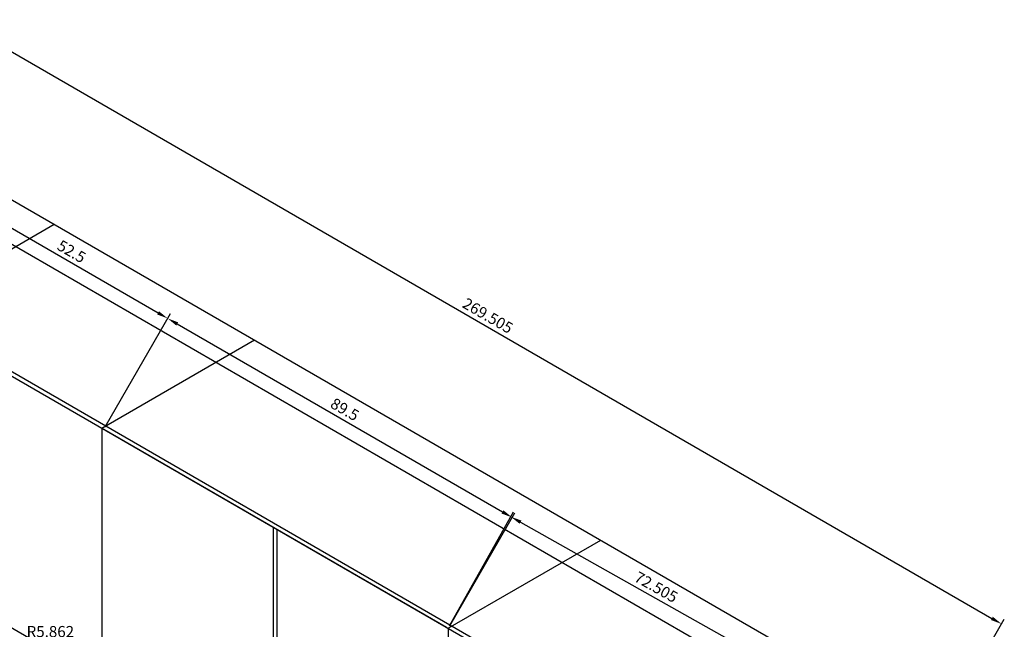
# Model space of a CAD drawing. Units: centimetres. Extents: x 239489 to 240034, y 95136 to 95693.
# Tile 4 of 4: x 239762 to 239984, y 95556 to 95693. Entities that reach past the tile are written whole.
import ezdxf

# ---------------------------------------------------------------- set-up
doc = ezdxf.new("R2010")
doc.units = ezdxf.units.CM
doc.layers.add('A-ANNO-DIMS', color=2, linetype='Continuous', lineweight=18)
doc.layers.add('A-FLOR-CASE', color=7, linetype='Continuous', lineweight=25)
doc.styles.get("Standard").update_dxf_attribs({"font": 'arial.ttf'})
doc.dimstyles.new('ISO-25', dxfattribs={"dimtxt": 2.5, "dimasz": 2.5, "dimexe": 1.25, "dimexo": 0.625, "dimtad": 1, "dimdec": 1, "dimdsep": 46, "dimtxsty": 'Standard', "dimcen": 2.5, "dimadec": 0, "dimazin": 0, "dimtfac": 1, "dimtdec": 1, "dimtmove": 0, "dimatfit": 3, "dimfxl": 1, "dimarcsym": 0})

# ---------------------------------------------------------------- blocks, each defined once
blk = doc.blocks.new('*D5')
at = {"layer": 'A-ANNO-DIMS', "color": 0, "lineweight": -2, "transparency": 16777216}
for p, q in [((239735.57, 95667.89), (239750.25, 95693.33)), ((239751.79, 95691), (239980.86, 95558.75)), ((239968.97, 95533.14), (239983.65, 95558.58))]:
    blk.add_line(p, q, dxfattribs=at)
at = {"layer": 'A-ANNO-DIMS', "color": 0, "transparency": 16777216}
for points in [[(239752, 95691.36), (239751.59, 95690.64), (239749.63, 95692.25)], [(239981.07, 95559.11), (239980.65, 95558.39), (239983.03, 95557.5)]]:
    blk.add_solid(points, dxfattribs=at)
at = {"layer": 'Defpoints', "color": 0, "transparency": 16777216}
for p in [(239735.25, 95667.35), (239983.03, 95557.5), (239968.65, 95532.6)]:
    blk.add_point(p, dxfattribs=at)
at = {"layer": 'A-ANNO-DIMS', "color": 0, "transparency": 16777216, "insert": (239867.28, 95626.52), "char_height": 2.5, "attachment_point": 5, "rotation": 330}
blk.add_mtext('269.505', dxfattribs=at)
blk = doc.blocks.new('*D22')
at = {"layer": 'A-ANNO-DIMS', "color": 0, "lineweight": -2, "transparency": 16777216}
for p, q in [((239735.88, 95628.07), (239750.57, 95653.51)), ((239752.11, 95651.18), (239793.24, 95627.43)), ((239781.35, 95601.82), (239796.03, 95627.26))]:
    blk.add_line(p, q, dxfattribs=at)
at = {"layer": 'A-ANNO-DIMS', "color": 0, "transparency": 16777216}
for points in [[(239752.32, 95651.54), (239751.9, 95650.82), (239749.94, 95652.43)], [(239793.45, 95627.79), (239793.04, 95627.07), (239795.41, 95626.18)]]:
    blk.add_solid(points, dxfattribs=at)
at = {"layer": 'Defpoints', "color": 0, "transparency": 16777216}
for p in [(239735.57, 95627.53), (239795.41, 95626.18), (239781.03, 95601.28)]:
    blk.add_point(p, dxfattribs=at)
at = {"layer": 'A-ANNO-DIMS', "color": 0, "transparency": 16777216, "insert": (239773.63, 95640.95), "char_height": 2.5, "attachment_point": 5, "rotation": 330}
blk.add_mtext('52.5', dxfattribs=at)
blk = doc.blocks.new('*D23')
at = {"layer": 'A-ANNO-DIMS', "color": 0, "lineweight": -2, "transparency": 16777216}
for p, q in [((239781.35, 95601.82), (239796.03, 95627.26)), ((239797.57, 95624.93), (239870.75, 95582.68)), ((239858.86, 95557.07), (239873.54, 95582.51))]:
    blk.add_line(p, q, dxfattribs=at)
at = {"layer": 'A-ANNO-DIMS', "color": 0, "transparency": 16777216}
for points in [[(239797.78, 95625.29), (239797.37, 95624.57), (239795.41, 95626.18)], [(239870.96, 95583.04), (239870.54, 95582.32), (239872.92, 95581.43)]]:
    blk.add_solid(points, dxfattribs=at)
at = {"layer": 'Defpoints', "color": 0, "transparency": 16777216}
for p in [(239781.03, 95601.28), (239872.92, 95581.43), (239858.54, 95556.53)]:
    blk.add_point(p, dxfattribs=at)
at = {"layer": 'A-ANNO-DIMS', "color": 0, "transparency": 16777216, "insert": (239835.11, 95605.45), "char_height": 2.5, "attachment_point": 5, "rotation": 330}
blk.add_mtext('89.5', dxfattribs=at)
blk = doc.blocks.new('*D24')
at = {"layer": 'A-ANNO-DIMS', "color": 0, "lineweight": -2, "transparency": 16777216}
for p, q in [((239858.85, 95557.08), (239873.23, 95582.69)), ((239874.8, 95580.37), (239933.66, 95547.32)), ((239922.07, 95521.58), (239936.45, 95547.19))]:
    blk.add_line(p, q, dxfattribs=at)
at = {"layer": 'A-ANNO-DIMS', "color": 0, "transparency": 16777216}
for points in [[(239875, 95580.74), (239874.6, 95580.01), (239872.62, 95581.6)], [(239933.86, 95547.69), (239933.46, 95546.96), (239935.84, 95546.1)]]:
    blk.add_solid(points, dxfattribs=at)
at = {"layer": 'Defpoints', "color": 0, "transparency": 16777216}
for p in [(239858.54, 95556.53), (239935.84, 95546.1), (239921.76, 95521.03)]:
    blk.add_point(p, dxfattribs=at)
at = {"layer": 'A-ANNO-DIMS', "color": 0, "transparency": 16777216, "insert": (239905.16, 95565.51), "char_height": 2.5, "attachment_point": 5, "rotation": 330.6844}
blk.add_mtext('72.505', dxfattribs=at)
blk = doc.blocks.new('*D39')
at = {"layer": 'A-ANNO-DIMS', "color": 0, "lineweight": -2, "transparency": 16777216}
for p, q in [((239717.29, 95549.03), (239731.97, 95574.47)), ((239733.51, 95572.13), (239765.51, 95553.66)), ((239753.61, 95528.06), (239768.3, 95553.5))]:
    blk.add_line(p, q, dxfattribs=at)
at = {"layer": 'A-ANNO-DIMS', "color": 0, "transparency": 16777216}
for points in [[(239733.72, 95572.5), (239733.31, 95571.77), (239731.35, 95573.38)], [(239765.72, 95554.02), (239765.3, 95553.3), (239767.67, 95552.41)]]:
    blk.add_solid(points, dxfattribs=at)
at = {"layer": 'Defpoints', "color": 0, "transparency": 16777216}
for p in [(239767.67, 95552.41), (239716.97, 95548.49), (239753.3, 95527.52)]:
    blk.add_point(p, dxfattribs=at)
at = {"layer": 'A-ANNO-DIMS', "color": 0, "transparency": 16777216, "insert": (239750.46, 95564.55), "char_height": 2.5, "attachment_point": 5, "rotation": 330}
blk.add_mtext('41.943', dxfattribs=at)
blk = doc.blocks.new('*D51')
at = {"layer": 'A-ANNO-DIMS', "color": 0, "lineweight": -2, "transparency": 16777216}
for p, q in [((239762.99, 95553.56), (239777.54, 95553.56)), ((239785.9, 95553.56), (239780.04, 95553.56))]:
    blk.add_line(p, q, dxfattribs=at)
at = {"layer": 'A-ANNO-DIMS', "color": 0, "transparency": 16777216}
blk.add_solid([(239777.54, 95553.98), (239777.54, 95553.15), (239780.04, 95553.56)], dxfattribs=at)
at = {"layer": 'Defpoints', "color": 0, "transparency": 16777216}
for p in [(239780.04, 95553.56), (239785.9, 95553.56)]:
    blk.add_point(p, dxfattribs=at)
at = {"layer": 'A-ANNO-DIMS', "color": 0, "transparency": 16777216, "insert": (239769.01, 95555.46), "char_height": 2.5, "attachment_point": 5, "rotation": 0.0036}
blk.add_mtext('R5.862', dxfattribs=at)

msp = doc.modelspace()

# ---------------------------------------------------------------- linework, layer by layer
at = {"layer": 'A-FLOR-CASE'}
for p, q in [((239735.2548, 95667.3502), (239968.6531, 95532.5976)), ((239735.2548, 95657.3502), (239947.431, 95534.8502)), ((239736.4333, 95628.0306), (239769.8958, 95647.3502)), ((239735.5673, 95628.5306), (239921.7628, 95521.0306)), ((239735.5673, 95627.5306), (239921.7628, 95520.0306)), ((239780.6006, 95601.5306), (239814.9291, 95621.3502)), ((239780.6006, 95601.5306), (239780.6006, 95538.5306)), ((239781.0336, 95601.2806), (239858.1099, 95556.7806)), ((239819.1388, 95579.2806), (239819.1388, 95533.8134)), ((239820.0048, 95578.7806), (239820.0048, 95533.3134)), ((239858.5429, 95556.5306), (239892.8714, 95576.3502)), ((239858.5429, 95556.5306), (239858.5429, 95493.5306))]:
    msp.add_line(p, q, dxfattribs=at)

# ---------------------------------------------------------------- dimensions: what is measured, and where the dimension line sits
at = {"layer": 'A-ANNO-DIMS'}
for base, p1, p2, angle, override, picture, middle in [((239983.0281, 95557.4959), (239735.2548, 95667.3502), (239968.6531, 95532.5976), 330, {"dimdec": 3, "dimlfac": 1, "dimrnd": 0, "dimzin": 0, "dimdsep": 46, "dimlunit": 2}, '*D5', (239867.2796, 95626.5188)), ((239795.4086, 95626.1788), (239735.5673, 95627.5306), (239781.0336, 95601.2806), 330, {"dimdec": 1, "dimlfac": 1, "dimrnd": 0, "dimzin": 0, "dimdsep": 46, "dimlunit": 2}, '*D22', (239773.6262, 95640.9505)), ((239872.9179, 95581.4288), (239781.0336, 95601.2806), (239858.5429, 95556.5306), 330, {"dimdec": 1, "dimlfac": 1, "dimrnd": 0, "dimzin": 0, "dimdsep": 46, "dimlunit": 2}, '*D23', (239835.114, 95605.4505)), ((239935.8394, 95546.0987), (239858.5429, 95556.5306), (239921.7628, 95521.0306), 330.684376, {"dimdec": 3, "dimlfac": 1, "dimrnd": 0, "dimzin": 0, "dimdsep": 46, "dimlunit": 2}, '*D24', (239905.1604, 95565.5067)), ((239767.673, 95552.4136), (239716.9746, 95548.4867), (239753.298, 95527.5153), 330, {"dimdec": 3, "dimlfac": 1, "dimrnd": 0, "dimzin": 0, "dimdsep": 46, "dimlunit": 2}, '*D39', (239750.4624, 95564.5466))]:
    dim = msp.add_linear_dim(base=base, p1=p1, p2=p2, angle=angle, dimstyle='ISO-25', override=override, dxfattribs=at)
    dim.commit()
    dim.dimension.update_dxf_attribs({"geometry": picture, "text_midpoint": middle})
dim = msp.add_radius_dim(center=(239785.9025, 95553.5634), mpoint=(239780.0408, 95553.563), dimstyle='ISO-25', override={"dimdec": 3, "dimlfac": 1, "dimrnd": 0, "dimzin": 0, "dimdsep": 46, "dimlunit": 2}, dxfattribs=at)
dim.commit()
dim.dimension.update_dxf_attribs({"geometry": '*D51', "text_midpoint": (239769.0141, 95555.4637)})

doc.saveas('drawing.dxf')
